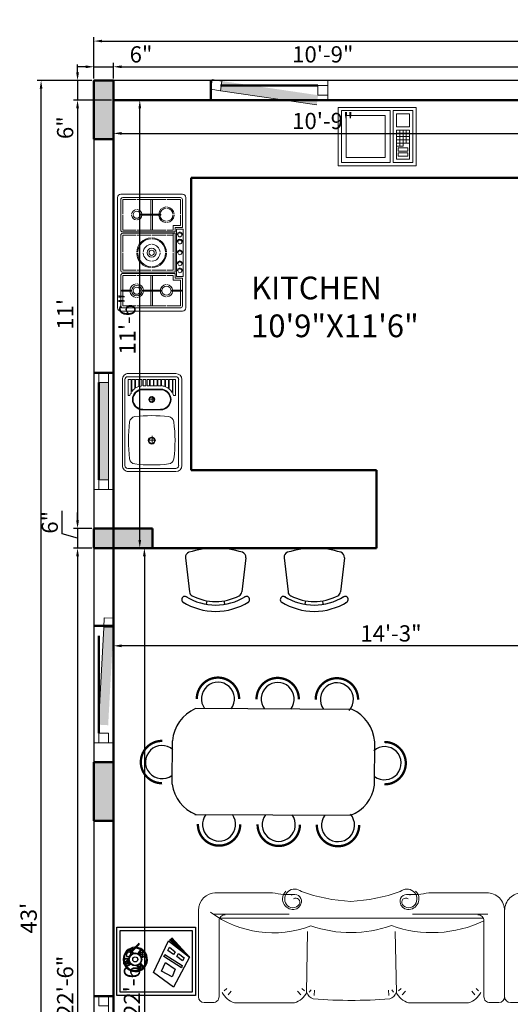
# Model space of a CAD drawing. Units: inches. Extents: x 3064 to 19385, y 846 to 15425.
# Tile 84 of 108: x 7077 to 7228, y 1112 to 1415. Entities that reach past the tile are written whole.
import ezdxf

# ---------------------------------------------------------------- set-up
doc = ezdxf.new("R2010")
doc.units = ezdxf.units.IN
for name, color, linetype, lineweight in [('A-ANNO-DIMS', 2, 'Continuous', 18), ('A-AREA-IDEN', 3, 'Continuous', 18), ('A-COLS', 1, 'Continuous', 35), ('A-EQPM', 8, 'Continuous', 18), ('A-FLOR-FIXT', 9, 'Continuous', 18), ('A-FURN', 8, 'Continuous', 18), ('A-GLAZ', 4, 'Continuous', 18), ('A-WALL', 7, 'Continuous', 50), ('C-PROP', 6, 'Continuous', 25)]:
    doc.layers.add(name, color=color, linetype=linetype, lineweight=lineweight)
for name, color, linetype in [('BLO', 135, 'Continuous'), ('FUR', 42, 'Continuous'), ('NOITHAT', 21, 'Continuous'), ('Win', 152, 'Continuous')]:
    doc.layers.add(name, color=color, linetype=linetype)
doc.styles.get("Standard").update_dxf_attribs({"font": 'arial.ttf'})
doc.dimstyles.new('ISO-25', dxfattribs={"dimtxt": 9, "dimasz": 2.5, "dimexe": 1.25, "dimexo": 0.625, "dimtad": 1, "dimdec": 1, "dimlunit": 3, "dimtxsty": 'Standard', "dimcen": 2.5, "dimadec": 0, "dimazin": 0, "dimtfac": 1, "dimtdec": 1, "dimtmove": 0, "dimatfit": 3, "dimfxl": 1, "dimarcsym": 0})

# ---------------------------------------------------------------- blocks, each defined once
blk = doc.blocks.new('*D291')
at = {"layer": 'A-ANNO-DIMS', "color": 0, "lineweight": -2, "transparency": 16777216}
for p, q in [((7099.71, 1396.96), (7099.71, 1401.84)), ((7105.71, 1396.96), (7105.71, 1401.84)), ((7097.21, 1400.59), (7094.71, 1400.59)), ((7099.71, 1400.59), (7105.71, 1400.59)), ((7108.21, 1400.59), (7117.73, 1400.59))]:
    blk.add_line(p, q, dxfattribs=at)
at = {"layer": 'A-ANNO-DIMS', "color": 0, "transparency": 16777216}
for points in [[(7097.21, 1401.01), (7097.21, 1400.18), (7099.71, 1400.59)], [(7108.21, 1401.01), (7108.21, 1400.18), (7105.71, 1400.59)]]:
    blk.add_solid(points, dxfattribs=at)
at = {"layer": 'Defpoints', "color": 0, "transparency": 16777216}
for p in [(7105.71, 1400.59), (7099.71, 1396.34), (7105.71, 1396.34)]:
    blk.add_point(p, dxfattribs=at)
at = {"layer": 'A-ANNO-DIMS', "color": 0, "transparency": 16777216, "insert": (7114.22, 1403.77), "char_height": 5, "attachment_point": 5}
blk.add_mtext('6"', dxfattribs=at)
blk = doc.blocks.new('*D292')
at = {"layer": 'A-ANNO-DIMS', "color": 0, "lineweight": -2, "transparency": 16777216}
for p, q in [((7105.71, 1396.96), (7105.71, 1401.84)), ((7234.71, 1396.96), (7234.71, 1401.84)), ((7108.21, 1400.59), (7232.21, 1400.59))]:
    blk.add_line(p, q, dxfattribs=at)
at = {"layer": 'A-ANNO-DIMS', "color": 0, "transparency": 16777216}
for points in [[(7108.21, 1401.01), (7108.21, 1400.18), (7105.71, 1400.59)], [(7232.21, 1401.01), (7232.21, 1400.18), (7234.71, 1400.59)]]:
    blk.add_solid(points, dxfattribs=at)
at = {"layer": 'Defpoints', "color": 0, "transparency": 16777216}
for p in [(7234.71, 1400.59), (7105.71, 1396.34), (7234.71, 1396.34)]:
    blk.add_point(p, dxfattribs=at)
at = {"layer": 'A-ANNO-DIMS', "color": 0, "transparency": 16777216, "insert": (7170.21, 1403.77), "char_height": 5, "attachment_point": 5}
blk.add_mtext('10\'-9"', dxfattribs=at)
blk = doc.blocks.new('*D296')
at = {"layer": 'A-ANNO-DIMS', "color": 0, "lineweight": -2, "transparency": 16777216}
for p, q in [((7094.68, 1398.84), (7094.68, 1401.34)), ((7099.08, 1396.34), (7093.43, 1396.34)), ((7094.68, 1396.34), (7094.68, 1390.34)), ((7105.08, 1390.34), (7093.43, 1390.34)), ((7094.68, 1387.84), (7094.68, 1378.32))]:
    blk.add_line(p, q, dxfattribs=at)
at = {"layer": 'A-ANNO-DIMS', "color": 0, "transparency": 16777216}
for points in [[(7094.26, 1398.84), (7095.09, 1398.84), (7094.68, 1396.34)], [(7094.26, 1387.84), (7095.09, 1387.84), (7094.68, 1390.34)]]:
    blk.add_solid(points, dxfattribs=at)
at = {"layer": 'Defpoints', "color": 0, "transparency": 16777216}
for p in [(7099.71, 1396.34), (7094.68, 1390.34), (7105.71, 1390.34)]:
    blk.add_point(p, dxfattribs=at)
at = {"layer": 'A-ANNO-DIMS', "color": 0, "transparency": 16777216, "insert": (7091.5, 1381.83), "char_height": 5, "attachment_point": 5, "rotation": 90}
blk.add_mtext('6"', dxfattribs=at)
blk = doc.blocks.new('*D297')
at = {"layer": 'A-ANNO-DIMS', "color": 0, "lineweight": -2, "transparency": 16777216}
for p, q in [((7105.08, 1390.34), (7093.43, 1390.34)), ((7094.68, 1387.84), (7094.68, 1260.84)), ((7099.08, 1258.34), (7093.43, 1258.34))]:
    blk.add_line(p, q, dxfattribs=at)
at = {"layer": 'A-ANNO-DIMS', "color": 0, "transparency": 16777216}
for points in [[(7094.26, 1387.84), (7095.09, 1387.84), (7094.68, 1390.34)], [(7094.26, 1260.84), (7095.09, 1260.84), (7094.68, 1258.34)]]:
    blk.add_solid(points, dxfattribs=at)
at = {"layer": 'Defpoints', "color": 0, "transparency": 16777216}
for p in [(7105.71, 1390.34), (7094.68, 1258.34), (7099.71, 1258.34)]:
    blk.add_point(p, dxfattribs=at)
at = {"layer": 'A-ANNO-DIMS', "color": 0, "transparency": 16777216, "insert": (7091.54, 1324.34), "char_height": 5, "attachment_point": 5, "rotation": 90}
blk.add_mtext("11'", dxfattribs=at)
blk = doc.blocks.new('*D298')
at = {"layer": 'A-ANNO-DIMS', "color": 0, "lineweight": -2, "transparency": 16777216}
for p, q in [((7089.94, 1256.76), (7089.94, 1263.79)), ((7094.68, 1260.84), (7094.68, 1263.34)), ((7094.68, 1255.34), (7089.94, 1256.76)), ((7099.08, 1258.34), (7093.43, 1258.34)), ((7094.68, 1258.34), (7094.68, 1252.34)), ((7094.68, 1258.34), (7094.68, 1252.34)), ((7099.08, 1252.34), (7093.43, 1252.34)), ((7094.68, 1249.84), (7094.68, 1247.34))]:
    blk.add_line(p, q, dxfattribs=at)
at = {"layer": 'A-ANNO-DIMS', "color": 0, "transparency": 16777216}
for points in [[(7094.26, 1260.84), (7095.09, 1260.84), (7094.68, 1258.34)], [(7094.26, 1249.84), (7095.09, 1249.84), (7094.68, 1252.34)]]:
    blk.add_solid(points, dxfattribs=at)
at = {"layer": 'Defpoints', "color": 0, "transparency": 16777216}
for p in [(7099.71, 1258.34), (7094.68, 1252.34), (7099.71, 1252.34)]:
    blk.add_point(p, dxfattribs=at)
at = {"layer": 'A-ANNO-DIMS', "color": 0, "transparency": 16777216, "insert": (7086.76, 1260.27), "char_height": 5, "attachment_point": 5, "rotation": 90}
blk.add_mtext('6"', dxfattribs=at)
blk = doc.blocks.new('*D299')
at = {"layer": 'A-ANNO-DIMS', "color": 0, "lineweight": -2, "transparency": 16777216}
for p, q in [((7099.08, 1252.34), (7093.43, 1252.34)), ((7094.68, 1249.84), (7094.68, 984.84)), ((7105.08, 982.34), (7093.43, 982.34))]:
    blk.add_line(p, q, dxfattribs=at)
at = {"layer": 'A-ANNO-DIMS', "color": 0, "transparency": 16777216}
for points in [[(7094.26, 1249.84), (7095.09, 1249.84), (7094.68, 1252.34)], [(7094.26, 984.84), (7095.09, 984.84), (7094.68, 982.34)]]:
    blk.add_solid(points, dxfattribs=at)
at = {"layer": 'Defpoints', "color": 0, "transparency": 16777216}
for p in [(7099.71, 1252.34), (7094.68, 982.34), (7105.71, 982.34)]:
    blk.add_point(p, dxfattribs=at)
at = {"layer": 'A-ANNO-DIMS', "color": 0, "transparency": 16777216, "insert": (7091.5, 1117.34), "char_height": 5, "attachment_point": 5, "rotation": 90}
blk.add_mtext('22\'-6"', dxfattribs=at)
blk = doc.blocks.new('*D303')
at = {"layer": 'A-ANNO-DIMS', "color": 0, "lineweight": -2, "transparency": 16777216}
for p, q in [((7099.08, 1396.34), (7082.19, 1396.34)), ((7083.44, 882.84), (7083.44, 1393.84)), ((7099.08, 880.34), (7082.19, 880.34))]:
    blk.add_line(p, q, dxfattribs=at)
at = {"layer": 'A-ANNO-DIMS', "color": 0, "transparency": 16777216}
for points in [[(7083.02, 1393.84), (7083.86, 1393.84), (7083.44, 1396.34)], [(7083.02, 882.84), (7083.86, 882.84), (7083.44, 880.34)]]:
    blk.add_solid(points, dxfattribs=at)
at = {"layer": 'Defpoints', "color": 0, "transparency": 16777216}
for p in [(7083.44, 1396.34), (7099.71, 1396.34), (7099.71, 880.34)]:
    blk.add_point(p, dxfattribs=at)
at = {"layer": 'A-ANNO-DIMS', "color": 0, "transparency": 16777216, "insert": (7080.26, 1138.34), "char_height": 5, "attachment_point": 5, "rotation": 90}
blk.add_mtext("43'", dxfattribs=at)
blk = doc.blocks.new('*D315')
at = {"layer": 'A-ANNO-DIMS', "color": 0, "lineweight": -2, "transparency": 16777216}
for p, q in [((7099.71, 1396.96), (7099.71, 1409.76)), ((7102.21, 1408.51), (7439.21, 1408.51)), ((7441.71, 1396.96), (7441.71, 1409.76))]:
    blk.add_line(p, q, dxfattribs=at)
at = {"layer": 'A-ANNO-DIMS', "color": 0, "transparency": 16777216}
for points in [[(7102.21, 1408.93), (7102.21, 1408.1), (7099.71, 1408.51)], [(7439.21, 1408.93), (7439.21, 1408.1), (7441.71, 1408.51)]]:
    blk.add_solid(points, dxfattribs=at)
at = {"layer": 'Defpoints', "color": 0, "transparency": 16777216}
for p in [(7441.71, 1408.51), (7099.71, 1396.34), (7441.71, 1396.34)]:
    blk.add_point(p, dxfattribs=at)
at = {"layer": 'A-ANNO-DIMS', "color": 0, "transparency": 16777216, "insert": (7270.71, 1411.69), "char_height": 5, "attachment_point": 5}
blk.add_mtext('28\'-6"', dxfattribs=at)
blk = doc.blocks.new('*D288')
at = {"layer": 'A-ANNO-DIMS', "color": 0, "lineweight": -2, "transparency": 16777216}
for p, q in [((7105.71, 1389.71), (7105.71, 1378.82)), ((7234.71, 1389.71), (7234.71, 1378.82)), ((7108.21, 1380.07), (7232.21, 1380.07))]:
    blk.add_line(p, q, dxfattribs=at)
at = {"layer": 'A-ANNO-DIMS', "color": 0, "transparency": 16777216}
for points in [[(7108.21, 1380.49), (7108.21, 1379.66), (7105.71, 1380.07)], [(7232.21, 1380.49), (7232.21, 1379.66), (7234.71, 1380.07)]]:
    blk.add_solid(points, dxfattribs=at)
at = {"layer": 'Defpoints', "color": 0, "transparency": 16777216}
for p in [(7105.71, 1390.34), (7234.71, 1390.34), (7234.71, 1380.07)]:
    blk.add_point(p, dxfattribs=at)
at = {"layer": 'A-ANNO-DIMS', "color": 0, "transparency": 16777216, "insert": (7170.21, 1383.25), "char_height": 5, "attachment_point": 5}
blk.add_mtext('10\'-9"', dxfattribs=at)
blk = doc.blocks.new('*D289')
at = {"layer": 'A-ANNO-DIMS', "color": 0, "lineweight": -2, "transparency": 16777216}
for p, q in [((7106.33, 1390.34), (7115.09, 1390.34)), ((7113.84, 1254.84), (7113.84, 1387.84)), ((7106.33, 1252.34), (7115.09, 1252.34))]:
    blk.add_line(p, q, dxfattribs=at)
at = {"layer": 'A-ANNO-DIMS', "color": 0, "transparency": 16777216}
for points in [[(7113.43, 1387.84), (7114.26, 1387.84), (7113.84, 1390.34)], [(7113.43, 1254.84), (7114.26, 1254.84), (7113.84, 1252.34)]]:
    blk.add_solid(points, dxfattribs=at)
at = {"layer": 'Defpoints', "color": 0, "transparency": 16777216}
for p in [(7105.71, 1390.34), (7113.84, 1390.34), (7105.71, 1252.34)]:
    blk.add_point(p, dxfattribs=at)
at = {"layer": 'A-ANNO-DIMS', "color": 0, "transparency": 16777216, "insert": (7110.67, 1321.34), "char_height": 5, "attachment_point": 5, "rotation": 90}
blk.add_mtext('11\'-6"', dxfattribs=at)
blk = doc.blocks.new('*D223')
at = {"layer": 'A-ANNO-DIMS', "color": 0, "lineweight": -2, "transparency": 16777216}
for p, q in [((7106.33, 1252.34), (7116.51, 1252.34)), ((7115.26, 1249.84), (7115.26, 984.84)), ((7106.33, 982.34), (7116.51, 982.34))]:
    blk.add_line(p, q, dxfattribs=at)
at = {"layer": 'A-ANNO-DIMS', "color": 0, "transparency": 16777216}
for points in [[(7114.84, 1249.84), (7115.67, 1249.84), (7115.26, 1252.34)], [(7114.84, 984.84), (7115.67, 984.84), (7115.26, 982.34)]]:
    blk.add_solid(points, dxfattribs=at)
at = {"layer": 'Defpoints', "color": 0, "transparency": 16777216}
for p in [(7105.71, 1252.34), (7105.71, 982.34), (7115.26, 982.34)]:
    blk.add_point(p, dxfattribs=at)
at = {"layer": 'A-ANNO-DIMS', "color": 0, "transparency": 16777216, "insert": (7112.08, 1117.34), "char_height": 5, "attachment_point": 5, "rotation": 90}
blk.add_mtext('22\'-6"', dxfattribs=at)
blk = doc.blocks.new('*D239')
at = {"layer": 'A-ANNO-DIMS', "color": 0, "lineweight": -2, "transparency": 16777216}
for p, q in [((7105.71, 1222.85), (7105.71, 1223.48)), ((7276.71, 1222.85), (7276.71, 1223.48)), ((7274.21, 1222.23), (7108.21, 1222.23))]:
    blk.add_line(p, q, dxfattribs=at)
at = {"layer": 'A-ANNO-DIMS', "color": 0, "transparency": 16777216}
for points in [[(7108.21, 1222.64), (7108.21, 1221.81), (7105.71, 1222.23)], [(7274.21, 1222.64), (7274.21, 1221.81), (7276.71, 1222.23)]]:
    blk.add_solid(points, dxfattribs=at)
at = {"layer": 'Defpoints', "color": 0, "transparency": 16777216}
for p in [(7105.71, 1222.23), (7105.71, 1222.23), (7276.71, 1222.23)]:
    blk.add_point(p, dxfattribs=at)
at = {"layer": 'A-ANNO-DIMS', "color": 0, "transparency": 16777216, "insert": (7191.21, 1225.4), "char_height": 5, "attachment_point": 5}
blk.add_mtext('14\'-3"', dxfattribs=at)
blk = doc.blocks.new('din')
at = {"layer": 'FUR', "ltscale": 0.25}
for p, q in [((70.23, 15.24), (9.28, 15.24)), ((0, 3.44), (0, -13.56)), ((79.14, 3.44), (79.14, -13.56)), ((8.91, -26.16), (70.23, -26.16))]:
    blk.add_line(p, q, dxfattribs=at)
at = {"layer": 'FUR', "ltscale": 0.25, "const_width": 0.9}
for points in [[(22.5, 19.02, 1.012537), (5.94, 19.02, 1.012537)], [(45.67, 19.02, 1.012537), (29.11, 19.02, 1.012537)], [(69.02, 19.02, 1.012537), (52.46, 19.02, 1.012537)], [(-3.79, 3.1, 1.012537), (-3.79, -13.47, 1.012537)], [(83.08, 3.1, -1.012537), (83.08, -13.47, -1.012537)], [(23.18, -29.95, -1.012537), (6.61, -29.95, -1.012537)], [(46.34, -29.95, -1.012537), (29.78, -29.95, -1.012537)], [(69.7, -29.95, -1.012537), (53.14, -29.95, -1.012537)]]:
    blk.add_lwpolyline(points, format="xyb", dxfattribs=at)
at = {"layer": 'FUR', "ltscale": 0.25}
for centre, radius, start, end in [((14.22, 19.13), 6.48, 323.1301, 221.2163), ((37.39, 19.13), 6.48, 323.1301, 216.8699), ((60.74, 19.13), 6.48, 323.1301, 216.8699), ((14.55, 1.54), 14.67, 111.0491, 172.5731), ((64.59, 1.54), 14.67, 7.4269, 68.9509), ((-3.89, -5.18), 6.48, 53.1301, 311.2163), ((83.18, -5.18), 6.48, 228.7837, 126.8699), ((15.28, -12.21), 15.34, 185.0602, 245.4675), ((63.86, -12.21), 15.34, 294.5325, 354.9398), ((14.89, -30.05), 6.48, 138.7837, 36.8699), ((38.06, -30.05), 6.48, 143.1301, 36.8699), ((61.42, -30.05), 6.48, 143.1301, 36.8699)]:
    blk.add_arc(centre, radius, start, end, dxfattribs=at)
blk = doc.blocks.new('A$C558E769F')
at = {"layer": 'NOITHAT'}
for p, q in [((29.4, 426.4), (61.1, 154.1)), ((508.9, 426.4), (477.2, 154.1)), ((197.1, 55.9), (201.8, 84.2)), ((341.2, 55.9), (336.5, 84.2))]:
    blk.add_line(p, q, dxfattribs=at)
for centre, radius, start, end in [((69.1, 431), 40, 107.02981, 186.63805), ((269.2, -222), 723, 72.97019, 107.02981), ((469.2, 431), 40, 353.36195, 72.97019), ((25.3, 93.7), 25.7, 44.80366, 252.32262), ((269.2, 492.6), 442.6, 237.77056, 302.22944), ((100.8, 158.7), 40, 186.63805, 243.24485), ((269.2, 492.6), 413.9, 243.24485, 296.75515), ((437.5, 158.7), 40, 296.75515, 353.36195), ((513, 93.7), 25.7, 287.67738, 135.19634), ((269.2, 492.6), 492.6, 237.85101, 302.14899)]:
    blk.add_arc(centre, radius, start, end, dxfattribs=at)
blk = doc.blocks.new('sofa-32')
at = {"color": 0, "linetype": 'ByBlock'}
for p, q in [((-0.026, 0.9238), (-0.1, 0.9238)), ((0.657, 0.9252), (0.1531, 0.9252)), ((1.6158, 0.9252), (2.1197, 0.9252)), ((2.3728, 0.9238), (2.2988, 0.9238)), ((-0.15, 0.15), (-0.15, 0.8738)), ((0.024, 0.2361), (0.024, 0.8738)), ((0.05, 0.8375), (0.05, 0.8379)), ((0.1006, 0.8574), (0.1265, 0.8286)), ((0.7096, 0.8574), (0.6837, 0.8286)), ((0.7682, 0.3257), (0.7597, 0.8384)), ((0.7601, 0.8375), (0.7601, 0.8379)), ((0.7823, 0.8346), (0.7966, 0.8162)), ((0.8227, 0.8633), (0.8259, 0.8195)), ((1.4501, 0.8633), (1.447, 0.8195)), ((1.4906, 0.8346), (1.4762, 0.8162)), ((1.5046, 0.3257), (1.5131, 0.8384)), ((1.5127, 0.8375), (1.5127, 0.8379)), ((1.5632, 0.8574), (1.5891, 0.8286)), ((2.1722, 0.8574), (2.1463, 0.8286)), ((2.2228, 0.8375), (2.2228, 0.8379)), ((2.2228, 0.8375), (2.2228, 0.8379)), ((2.2488, 0.2361), (2.2488, 0.8738)), ((2.4228, 0.15), (2.4228, 0.8738)), ((0.0903, 0.8062), (0.0682, 0.8242)), ((0.7199, 0.8062), (0.742, 0.8242)), ((1.5529, 0.8062), (1.5308, 0.8242)), ((2.1825, 0.8062), (2.2046, 0.8242)), ((-0.01, 0.1801), (0.6238, 0.1801)), ((0.0289, 0.2145), (2.2439, 0.2145)), ((2.2948, 0.1801), (1.661, 0.1801)), ((0, 0), (0.4856, 0)), ((2.2848, 0), (1.7991, 0))]:
    blk.add_line(p, q, dxfattribs=at)
at = {"color": 0, "linetype": 'ByBlock', "extrusion": (0, 0, -1)}
for centre, major_axis, start_param, end_param in [((-0.1, 0.8738), (0.0354, 0.0354), 3.926992, 5.497787), ((-0.026, 0.8738), (-0.0354, 0.0354), 0.785398, 2.356196), ((0.1997, 0.7661), (0.1173, 0.1173), 4.372209, 5.213218), ((0.6105, 0.7661), (0.1173, 0.1173), -0.500829, 0.34018), ((1.6624, 0.7661), (0.1173, 0.1173), 4.372209, 5.213218), ((2.0731, 0.7661), (-0.1173, 0.1173), 1.069968, 1.910976), ((2.2988, 0.8738), (-0.0354, 0.0354), 5.497786, 7.068583), ((2.3728, 0.8738), (0.0354, 0.0354), -0.785398, 0.785398), ((0.8378, 0.8143), (-0.0573, 0.0573), 5.78837, 6.779907), ((1.1202, -2.7856), (2.6094, 2.6094), -0.86827, -0.778364), ((1.1526, -2.7856), (2.6094, 2.6094), -0.792432, -0.702526), ((1.435, 0.8143), (-0.0573, 0.0573), 1.074075, 2.065611), ((0.4599, -0.6685), (0.71, 0.71), 5.048761, 5.844539), ((1.1424, -0.6685), (-0.71, 0.71), 0.438646, 1.125824), ((1.7954, -0.5466), (-0.6249, 0.6249), 0.417642, 1.423136), ((0.074, 0.2361), (0.0354, 0.0354), 2.356194, 3.926992), ((2.1988, 0.2361), (0.0354, 0.0354), 0.785397, 2.356194), ((0, 0.15), (0.1061, 0.1061), 2.356194, 3.926992), ((0.6576, 0.0525), (-0.0624, 0.0624), 4.675944, 7.152385), ((0.6708, 0.0524), (-0.059, 0.059), 3.186406, 6.094039), ((0.6552, 0.0629), (0.0458, 0.0458), 4.523242, 6.472337), ((0.6801, 0.0798), (-0.0245, 0.0245), 1.759948, 4.523241), ((0.6592, 0.0712), (-0.0491, 0.0491), 0.8692, 2.230507), ((1.6256, 0.0712), (-0.0491, 0.0491), 5.623477, 6.984784), ((1.614, 0.0524), (0.059, 0.059), 0.189149, 3.096782), ((1.6047, 0.0798), (0.0245, 0.0245), 1.759947, 4.52324), ((1.6295, 0.0629), (0.0458, 0.0458), 4.52324, 6.472335), ((1.6271, 0.0525), (-0.0624, 0.0624), 0.701599, 3.17804), ((2.2728, 0.15), (0.1061, 0.1061), 0.785398, 2.356194), ((0.6324, -0.6613), (-0.479, 0.479), 0.566947, 0.842011), ((0.6701, 0.0726), (0.0414, 0.0414), 0.659711, 2.852687), ((1.2153, -1.3904), (1.0359, 1.0359), 5.158011, 5.447964), ((1.0694, -1.3904), (1.0359, 1.0359), 5.547613, 5.837566), ((1.6147, 0.0726), (-0.0414, 0.0414), 3.430501, 5.623477), ((1.6523, -0.6613), (0.479, 0.479), 5.441177, 5.716241)]:
    blk.add_ellipse(centre, major_axis=major_axis, ratio=1, start_param=start_param, end_param=end_param, dxfattribs=at)
blk = doc.blocks.new('sofa-34')
at = {"color": 0, "linetype": 'ByBlock'}
for p, q in [((-0.026, 0.9238), (-0.1, 0.9238)), ((0.657, 0.9252), (0.1531, 0.9252)), ((0.8361, 0.9238), (0.9101, 0.9238)), ((-0.15, 0.15), (-0.15, 0.8738)), ((0.024, 0.2361), (0.024, 0.8738)), ((0.05, 0.8375), (0.05, 0.8379)), ((0.1006, 0.8574), (0.1265, 0.8286)), ((0.7096, 0.8574), (0.6837, 0.8286)), ((0.7601, 0.8375), (0.7601, 0.8379)), ((0.7602, 0.8375), (0.7601, 0.8379)), ((0.7861, 0.2361), (0.7861, 0.8738)), ((0.9601, 0.15), (0.9601, 0.8738)), ((0.0903, 0.8062), (0.0682, 0.8242)), ((0.7199, 0.8062), (0.742, 0.8242)), ((-0.01, 0.1801), (0.2738, 0.1801)), ((0.0289, 0.2145), (0.7812, 0.2145)), ((0.8201, 0.1801), (0.5364, 0.1801))]:
    blk.add_line(p, q, dxfattribs=at)
blk.add_arc((0.4051, 0.1479), 0.2579, 40.79835, 139.20165, dxfattribs=at)
at = {"color": 0, "linetype": 'ByBlock', "extrusion": (0, 0, -1)}
for centre, major_axis, ratio, start_param, end_param in [((-0.1, 0.8738), (0.0354, 0.0354), 1, 3.926992, 5.497787), ((-0.026, 0.8738), (-0.0354, 0.0354), 1, 0.785398, 2.356196), ((0.1997, 0.7661), (0.1173, 0.1173), 1, 4.372209, 5.213218), ((0.6105, 0.7661), (0.1173, 0.1173), 1, -0.500829, 0.34018), ((0.5004, -0.5869), (-0.4145, 0.931), 0.264583, -0.381915, 0.387685), ((0.074, 0.2361), (-0.0354, 0.0354), 1, 3.926991, 5.497788), ((0, 0.15), (0.1061, 0.1061), 1, 2.356194, 3.926992), ((0.1167, 0.0525), (-0.0624, 0.0624), 1, 4.675944, 7.152385), ((0.1299, 0.0524), (-0.059, 0.059), 1, 3.186406, 6.094039), ((0.1144, 0.0629), (-0.0458, 0.0458), 1, 6.094039, 8.043134), ((0.1392, 0.0798), (0.0245, 0.0245), 1, 0.189152, 2.952444), ((0.1183, 0.0712), (0.0491, 0.0491), 1, -0.701597, 0.659711), ((0.179, -0.6576), (-0.2506, 0.635), 0.885019, 0.124301, 0.339591), ((0.1292, 0.0726), (-0.0414, 0.0414), 1, 2.230507, 4.423483), ((0.3517, -0.5578), (0.7346, 0.1067), 0.76838, 4.597815, 5.20076)]:
    blk.add_ellipse(centre, major_axis=major_axis, ratio=ratio, start_param=start_param, end_param=end_param, dxfattribs=at)
at = {"color": 0, "linetype": 'ByBlock'}
for centre, major_axis, ratio, start_param, end_param in [((0.8361, 0.8738), (0.0354, 0.0354), 1, 0.785398, 2.356196), ((0.9101, 0.8738), (-0.0354, 0.0354), 1, 3.926992, 5.497787), ((0.3097, -0.5869), (0.4145, 0.931), 0.264583, -0.381915, 0.387685), ((0.7361, 0.2361), (0.0354, 0.0354), 1, 3.926991, 5.497788), ((0.6918, 0.0712), (-0.0491, 0.0491), 1, -0.701597, 0.659711), ((0.6802, 0.0524), (0.059, 0.059), 1, 3.186406, 6.094039), ((0.6709, 0.0798), (-0.0245, 0.0245), 1, 0.189152, 2.952444), ((0.6958, 0.0629), (0.0458, 0.0458), 1, 6.094039, 8.043134), ((0.6934, 0.0525), (0.0624, 0.0624), 1, 4.675944, 7.152385), ((0.8101, 0.15), (-0.1061, 0.1061), 1, 2.356194, 3.926992), ((0.6809, 0.0726), (0.0414, 0.0414), 1, 2.230507, 4.423483), ((0.6312, -0.6576), (0.2506, 0.635), 0.885019, 0.124301, 0.339591)]:
    blk.add_ellipse(centre, major_axis=major_axis, ratio=ratio, start_param=start_param, end_param=end_param, dxfattribs=at)
blk = doc.blocks.new('sink 1')
for points in [[(-7.34, 1.48), (-7.34, 22.73)], [(-6.56, 1.48), (-6.56, 22.73)], [(5.86, 24.22), (-5.86, 24.22)], [(6.01, 23.43), (-5.86, 23.43)], [(6.72, 1.48), (6.72, 22.73)], [(7.34, 1.48), (7.34, 22.73)], [(0, 15.39), (0, 17.42)], [(1.09, 16.48), (-0.94, 16.48)], [(-2.09, 8.99), (2.28, 8.99)], [(-2.09, 8.84), (2.28, 8.84)], [(-5.78, 5.39), (-5.78, 5.39)], [(-5.31, 5.39), (-5.31, 5.39)], [(-5.16, 4.92), (-5.16, 4.92)], [(0.78, 6.33), (-0.78, 6.33)], [(0, 5.55), (0, 7.26)], [(5.16, 4.92), (5.16, 4.92)], [(5.94, 5.39), (5.94, 5.39)], [(-5, 1.48), (-5, 4.69)], [(-5, 1.48), (-4.22, 1.48), (-4.22, 3.83)], [(-4.84, 4.45), (-4.84, 4.45)], [(-4.22, 3.83), (-4.22, 3.83)], [(-4.06, 1.48), (-4.06, 3.69)], [(-4.06, 1.48), (-3.28, 1.48), (-3.28, 3.27)], [(-3.91, 3.52), (-3.91, 3.52)], [(-3.28, 3.2), (-3.28, 3.2)], [(-3.12, 3.2), (-3.12, 3.2)], [(-2.34, 3.05), (-2.34, 3.05)], [(-2.19, 3.05), (-2.19, 3.05)], [(-2.09, 3.99), (2.28, 3.99)], [(-2.09, 3.84), (2.28, 3.84)], [(-1.41, 3.05), (-1.41, 3.05)], [(-1.25, 3.05), (-1.25, 3.05)], [(-0.47, 1.48), (-1.25, 1.48), (-1.25, 3.05), (-0.47, 3.05)], [(-0.62, 3.05), (-0.62, 3.05)], [(-0.47, 1.48), (-0.47, 3.05)], [(-0.31, 3.05), (-0.31, 3.05)], [(0.47, 1.48), (-0.31, 1.48), (-0.31, 3.05), (0.47, 3.05)], [(0.31, 3.05), (0.31, 3.05)], [(0.47, 1.48), (0.47, 3.05)], [(0.62, 3.05), (0.62, 3.05)], [(1.25, 3.05), (1.25, 3.05)], [(1.56, 3.05), (1.56, 3.05)], [(2.19, 3.05), (2.19, 3.05)], [(2.5, 3.05), (2.5, 3.05)], [(3.12, 3.2), (3.12, 3.2)], [(3.28, 1.48), (4.06, 1.48), (4.06, 3.57)], [(3.28, 1.48), (3.28, 3.2)], [(3.44, 3.2), (3.44, 3.2)], [(4.06, 3.52), (4.06, 3.52)], [(4.22, 1.48), (4.22, 3.67)], [(4.37, 3.83), (4.37, 3.83)], [(5, 4.45), (5, 4.45)], [(6.01, 0.78), (-5.86, 0.78)], [(5.86, 0), (-5.86, 0)], [(-5.78, 1.48), (-5.78, 1.48)], [(-5.16, 1.48), (-5.16, 1.48)], [(-4.84, 1.48), (-4.84, 1.48)], [(-4.22, 1.48), (-4.22, 1.48)], [(-3.91, 1.48), (-3.91, 1.48)], [(-3.28, 1.48), (-3.28, 1.48)], [(-3.12, 1.48), (-3.12, 1.48)], [(-2.34, 1.48), (-2.34, 1.48)], [(-2.19, 1.48), (-2.19, 1.48)], [(-1.41, 1.48), (-1.41, 1.48)], [(-1.25, 1.48), (-1.25, 1.48)], [(-0.62, 1.48), (-0.62, 1.48)], [(-0.31, 1.48), (-0.31, 1.48)], [(0.31, 1.48), (0.31, 1.48)], [(0.62, 1.48), (0.62, 1.48)], [(1.25, 1.48), (1.25, 1.48)], [(1.56, 1.48), (1.56, 1.48)], [(2.19, 1.48), (2.19, 1.48)], [(2.5, 1.48), (2.5, 1.48)], [(3.12, 1.48), (3.12, 1.48)], [(3.44, 1.48), (3.44, 1.48)], [(4.06, 1.48), (4.06, 1.48)], [(4.37, 1.48), (4.37, 1.48)], [(5, 1.48), (5, 1.48)], [(5.16, 1.48), (5.16, 1.48)], [(5.94, 1.48), (5.94, 1.48)]]:
    blk.add_lwpolyline(points)
for points in [[(-5.16, 4.92), (-5.16, 1.48), (-5.78, 1.48), (-5.78, 5.39), (-5.31, 5.39, -0.068511), (-5.16, 4.92)], [(5.16, 4.92, 0.248301), (5.47, 5.39), (5.94, 5.39), (5.94, 1.48), (5.16, 1.48), (5.16, 4.92)], [(4.06, 3.57, -0.061679), (3.32, 3.22)], [(4.22, 1.48), (5, 1.48), (5, 4.45, -0.083542), (4.22, 3.67, -0.083542)]]:
    blk.add_lwpolyline(points, format="xyb")
for points in [[(-3.12, 3.22), (-3.12, 1.48), (-2.34, 1.48), (-2.34, 3.05, -0.06228)], [(2.5, 3.05), (2.5, 1.48), (3.12, 1.48), (3.12, 3.2, -0.050256)]]:
    blk.add_lwpolyline(points, format="xyb", close=True)
for points in [[(-2.19, 3.05), (-1.41, 3.05), (-1.41, 1.48), (-2.19, 1.48)], [(0.62, 3.05), (1.25, 3.05), (1.25, 1.48), (0.62, 1.48)], [(2.19, 1.48), (2.19, 3.05), (1.56, 3.05), (1.56, 1.48)]]:
    blk.add_lwpolyline(points, close=True)
for centre, radius in [((0.09, 16.57), 0.859), ((0.09, 16.57), 0.703), ((0.09, 6.41), 0.703), ((0.09, 6.41), 0.547)]:
    blk.add_circle(centre, radius)
for centre, radius, start, end in [((-5.86, 22.73), 1.48, 90, 180), ((-5.86, 22.73), 0.703, 90, 180), ((-3.87, 20.82), 1.53, 97.3256, 171.1849), ((0.09, -12.65), 35.23, 83.2159, 96.7841), ((4.06, 20.82), 1.53, 8.8151, 82.6744), ((5.86, 22.73), 1.48, 360, 90), ((6.01, 22.73), 0.703, 0, 90), ((30.19, 16.56), 35.85, 172.7947, 187.4213), ((-30, 16.56), 35.85, 352.5787, 7.2053), ((-3.89, 12.12), 1.48, 187.4212, 263.2159), ((0.09, 45.63), 35.23, 263.2159, 276.7841), ((4.08, 12.12), 1.48, 276.7841, 352.5788), ((-2.1, 6.41), 2.58, 90, 270), ((-2.1, 6.41), 2.42, 90, 270), ((2.28, 6.41), 2.58, 270, 90), ((2.28, 6.41), 2.42, 270, 90), ((-2.15, 6.48), 3.36, 212.1095, 232.0862), ((-2.1, 6.41), 3.36, 234.156, 249.3275), ((2.14, 6.36), 3.36, 289.8633, 290.5971), ((-5.86, 1.48), 1.48, 180, 270), ((-5.86, 1.48), 0.703, 180, 270), ((5.86, 1.48), 1.48, 270, 0), ((6.01, 1.48), 0.703, 270, 360)]:
    blk.add_arc(centre, radius, start, end)
blk = doc.blocks.new('STOVE')
for p, q in [((11.85, 19.7), (11.55, 19.7)), ((11.55, 16.92), (11.55, 19.7)), ((11.85, 16.92), (11.85, 19.7)), ((11.85, 16.92), (11.55, 16.92)), ((-11.85, 13.73), (-11.85, 7.62)), ((-11.85, 13.73), (-11.55, 13.73)), ((-11.55, 13.73), (-11.55, 7.62)), ((11.85, 13.23), (11.55, 13.23)), ((11.55, 13.23), (11.55, 7.57)), ((11.85, 13.23), (11.85, 7.57)), ((-11.85, 10.75), (-16.4, 10.75)), ((-11.85, 10.25), (-16.4, 10.25)), ((-7, 10.75), (-11.55, 10.75)), ((-7, 10.25), (-11.55, 10.25)), ((7, 10.75), (11.55, 10.75)), ((7, 10.25), (11.55, 10.25)), ((11.85, 10.75), (16.4, 10.75)), ((11.85, 10.25), (16.4, 10.25)), ((-11.85, 7.62), (-11.55, 7.62)), ((11.85, 7.57), (11.55, 7.57)), ((-7, 3.9), (-8.4, 3.9)), ((-7.8, 3.3), (-7.8, 1)), ((-6.4, 3.3), (-7.8, 3.3)), ((-5.4, 3.9), (-6, 3.9)), ((-5.4, 3.9), (-0.15, 3.9)), ((0.15, 3.9), (5.4, 3.9)), ((6.4, 3.3), (7.8, 3.3)), ((7, 3.9), (8.4, 3.9)), ((7.8, 3.3), (7.8, 1)), ((8.4, 3.9), (8.4, 1.6)), ((11.85, 4.28), (11.55, 4.28)), ((11.55, 4.28), (11.55, 1.3)), ((11.85, 4.28), (11.85, 1.3)), ((7.3, 2.8), (-7.3, 2.8)), ((-7.3, 2.8), (-7.3, 0.8)), ((7.3, 0.8), (-7.3, 0.8)), ((7.3, 2.8), (7.3, 0.8)), ((11.85, 1.3), (11.55, 1.3))]:
    blk.add_line(p, q)
for points in [[(-17, 21), (17, 21, -0.414214), (18, 20), (18, 1, -0.414214), (17, 0), (-17, 0, -0.414214), (-18, 1), (-18, 20, -0.414214)], [(6, 3.3), (-6, 3.3), (-6, 19.4, -0.414214), (-5.4, 20), (5.4, 20, -0.414214), (6, 19.4)]]:
    blk.add_lwpolyline(points, format="xyb", close=True)
for points in [[(-7.8, 1), (-16.4, 1, -0.414214), (-17, 1.6), (-17, 19.4, -0.414214), (-16.4, 20), (-7, 20, -0.414214), (-6.4, 19.4), (-6.4, 3.3)], [(6.4, 19.4, -0.414214), (7, 20), (16.4, 20, -0.414214), (17, 19.4), (17, 1.6, -0.414214), (16.4, 1), (7.8, 1)]]:
    blk.add_lwpolyline(points, format="xyb")
for points in [[(-16.4, 15.22), (-16.4, 19.4), (-11.85, 19.4)], [(-11.55, 19.4), (-7, 19.4), (-7, 15.22)], [(-5.4, 15.22), (-5.4, 19.4), (-0.15, 19.4)], [(0.15, 19.4), (5.4, 19.4), (5.4, 15.22)], [(6.4, 3.3), (6.4, 19.4)], [(7, 15.22), (7, 19.4), (11.55, 19.4)], [(11.85, 19.4), (16.4, 19.4), (16.4, 15.22)], [(-16.4, 6.08), (-16.4, 14.92)], [(-7, 14.92), (-7, 6.08)], [(-5.4, 10.65), (-5.4, 14.92)], [(5.4, 14.92), (5.4, 10.65)], [(7, 6.08), (7, 14.92)], [(16.4, 14.92), (16.4, 6.08)], [(-5.4, 6.08), (-5.4, 10.35)], [(5.4, 10.35), (5.4, 6.08)], [(-11.85, 1.6), (-16.4, 1.6), (-16.4, 5.77)], [(-8.4, 3.9), (-8.4, 1.6), (-11.55, 1.6)], [(-7, 5.77), (-7, 3.9)], [(-5.4, 3.9), (-5.4, 5.77)], [(5.4, 5.77), (5.4, 3.9)], [(7, 3.9), (7, 5.77)], [(16.4, 5.77), (16.4, 1.6), (11.85, 1.6)], [(11.55, 1.6), (8.4, 1.6)]]:
    blk.add_lwpolyline(points)
for centre, radius in [((-11.7, 15.07), 1.1), ((11.7, 15.07), 1.6), ((11.7, 15.07), 1.1), ((0, 10.5), 1.4), ((0, 10.5), 0.8), ((11.7, 5.93), 1.4), ((-5.49, 1.8), 0.6), ((-3.3, 1.8), 0.6), ((0, 1.8), 0.6), ((3.39, 1.8), 0.6), ((5.57, 1.8), 0.6)]:
    blk.add_circle(centre, radius)
for centre, radius, start, end in [((-11.7, 15.07), 1.6, 95.3794, 174.6206), ((-11.7, 15.07), 1.6, 5.3794, 84.6206), ((11.7, 15.07), 2.1, 94.096, 175.904), ((11.7, 15.07), 2.1, 4.096, 85.904), ((-11.7, 15.07), 1.6, 185.3794, 264.6206), ((-11.7, 15.07), 1.6, 275.3794, 354.6206), ((0, 10.5), 4.6, 91.8687, 178.1313), ((0, 10.5), 4.3, 91.9991, 178.0009), ((0, 10.5), 2.6, 93.3074, 176.6926), ((0, 10.5), 4.6, 1.8687, 88.1313), ((0, 10.5), 4.3, 1.9991, 88.0009), ((0, 10.5), 2.6, 3.3074, 86.6926), ((11.7, 15.07), 2.1, 184.096, 265.904), ((11.7, 15.07), 2.1, 274.096, 355.904), ((0, 10.5), 4.6, 181.8687, 268.1313), ((0, 10.5), 4.3, 181.9991, 268.0009), ((0, 10.5), 2.6, 183.3074, 266.6926), ((0, 10.5), 4.6, 271.8687, 358.1313), ((0, 10.5), 4.3, 271.9991, 358.0009), ((0, 10.5), 2.6, 273.3074, 356.6926), ((-11.7, 5.93), 2.4, 93.5833, 176.4167), ((-11.7, 5.93), 2, 94.3012, 175.6988), ((-11.7, 5.93), 2.4, 3.5833, 86.4167), ((-11.7, 5.93), 2, 4.3012, 85.6988), ((11.7, 5.93), 1.9, 94.5281, 175.4719), ((11.7, 5.93), 1.9, 4.5281, 85.4719), ((-11.7, 5.93), 2.4, 183.5833, 266.4167), ((-11.7, 5.93), 2, 184.3012, 265.6988), ((-11.7, 5.93), 2.4, 273.5833, 356.4167), ((-11.7, 5.93), 2, 274.3012, 355.6988), ((11.7, 5.93), 1.9, 184.5281, 265.4719), ((11.7, 5.93), 1.9, 274.5281, 355.4719), ((-5.49, 1.8), 0.846, 89.9979, 270), ((-3.3, 1.8), 0.846, 89.9979, 270), ((0, 1.8), 0.846, 89.9979, 270), ((3.39, 1.8), 0.846, 89.9979, 270), ((5.57, 1.8), 0.846, 89.9979, 270)]:
    blk.add_arc(centre, radius, start, end)
blk = doc.blocks.new('Microwave')
for p, q in [((18, 10), (22, 10)), ((19, 7), (19, 11)), ((20, 11), (20, 7)), ((21, 7), (21, 11)), ((22, 9), (18, 9)), ((18, 8), (22, 8)), ((22, 7), (18, 7)), ((19, 6), (19, 7)), ((20, 7), (20, 6)), ((20, 6), (18, 6))]:
    blk.add_line(p, q)
for points in [[(0, 0), (0, 18), (24, 18), (24, 0)], [(1, 1), (1, 17), (16, 17), (16, 1)], [(2.5, 2.5), (2.5, 15.5), (14.5, 15.5), (14.5, 2.5)], [(17, 1), (17, 17), (23, 17), (23, 1)], [(18, 12), (18, 16), (22, 16), (22, 12)], [(18, 2), (18, 11), (22, 11), (22, 2)], [(18.5, 4.5), (18.5, 5.5), (21.5, 5.5), (21.5, 4.5)], [(18.5, 3), (18.5, 4), (21.5, 4), (21.5, 3)]]:
    blk.add_lwpolyline(points, close=True)
blk = doc.blocks.new('ST1')
at = {"layer": 'BLO'}
for p, q in [((2.87, 1.65), (2.87, 24.72)), ((2.87, 24.72), (22.87, 24.72)), ((3.87, 2.65), (3.87, 23.72)), ((3.87, 23.72), (21.87, 23.72)), ((21.87, 23.72), (21.87, 2.65)), ((22.87, 24.72), (22.87, 1.65)), ((22.87, 1.65), (2.87, 1.65)), ((21.87, 2.65), (3.87, 2.65))]:
    blk.add_line(p, q, dxfattribs=at)
at = {"layer": 'Win'}
for p, q in [((11.4, 21.86), (12.09, 20.65)), ((11.51, 21.94), (12.19, 20.74)), ((11.57, 21.85), (13.19, 21.3)), ((12.55, 22.44), (12.13, 20.85)), ((12.55, 22.44), (13.25, 21.19)), ((12.69, 22.48), (13.4, 21.2)), ((14.51, 20.87), (14.54, 20.9)), ((14.64, 20.77), (14.67, 20.79)), ((15.43, 20.61), (15.22, 19.97)), ((15.22, 19.97), (15.71, 20.33)), ((15.27, 19.81), (15.82, 20.21)), ((15.37, 21.5), (15.64, 21.7)), ((15.41, 20.64), (17.8, 18.17)), ((15.46, 21.36), (15.76, 21.58)), ((15.54, 20.8), (16.34, 20.79)), ((15.54, 20.77), (18.02, 18.4)), ((15.76, 21.58), (15.55, 20.96)), ((17.88, 18.31), (15.58, 20.6)), ((15.87, 20.45), (16.34, 20.79)), ((15.99, 20.33), (16.41, 20.64)), ((10.46, 17.93), (11.6, 18.76)), ((10.53, 17.78), (11.65, 18.59)), ((10.53, 17.78), (12.23, 17.8)), ((11.59, 18.54), (11.11, 16.99)), ((11.11, 16.99), (12.23, 17.8)), ((11.23, 16.87), (12.37, 17.7)), ((13.9, 17.44), (14.58, 16.23)), ((14.03, 17.48), (14.71, 16.28)), ((14.09, 17.38), (15.67, 16.91)), ((15.04, 18.04), (14.71, 16.28)), ((14.97, 18.16), (15.67, 16.91)), ((15, 18.22), (15.87, 17.69)), ((15.13, 18.43), (16.01, 17.9)), ((15.14, 18.13), (15.77, 17.01)), ((5.28, 8.07), (9.58, 13.93)), ((8.3, 8.54), (10.02, 11.57)), ((9.58, 13.93), (18.91, 9.59)), ((10.02, 11.57), (12.5, 10.4)), ((12.5, 10.4), (10.58, 7.59)), ((10.98, 5.74), (14.34, 10.89)), ((14.87, 10.68), (11.67, 5.58)), ((18.91, 9.59), (14.09, 3.45)), ((14.09, 3.45), (19.17, 9.31)), ((14.09, 3.45), (19.44, 9.01)), ((14.09, 3.45), (19.64, 8.8)), ((14.34, 10.89), (14.87, 10.68)), ((14.86, 8.07), (16.06, 9.73)), ((17.01, 9.23), (15.7, 7.6)), ((16.06, 9.73), (17.01, 9.23)), ((14.09, 3.45), (5.28, 8.07)), ((10.58, 7.59), (8.3, 8.54)), ((13.06, 5.5), (14.27, 7.16)), ((15.21, 6.66), (13.91, 5.03)), ((14.09, 3.45), (19.77, 8.63)), ((14.27, 7.16), (15.21, 6.66)), ((15.7, 7.6), (14.86, 8.07)), ((11.67, 5.58), (10.98, 5.74)), ((13.91, 5.03), (13.06, 5.5))]:
    blk.add_line(p, q, dxfattribs=at)
for radius in [1.91, 1.75, 0.74]:
    blk.add_circle((13.43, 19.29), radius, dxfattribs=at)
for centre, radius, start, end in [((13.43, 19.29), 3.56, 1.5005, 355.5882), ((13.43, 19.29), 3.27, 6.8421, 0.252), ((15.21, 21.57), 0.956, 171.718, 281.8824), ((14.47, 21.69), 0.203, 96.3605, 174.3012), ((14.6, 20.95), 0.956, 349.0729, 98.9437), ((15.51, 20.66), 0.106, 78.1124, 194.2793), ((15.97, 17.77), 0.128, 220.7943, 60.0122), ((17.91, 18.29), 0.161, 227.8642, 43.7153)]:
    blk.add_arc(centre, radius, start, end, dxfattribs=at)
blk = doc.blocks.new('WIN-900-A')
h = blk.add_hatch(color=256)
h.dxf.hatch_style = 1
h.paths.add_polyline_path([(33, 0), (33, 3), (3, 3), (3, 0)])
blk.add_line((3, 0), (33, 0))
blk.add_lwpolyline([(3, 0), (0, 0), (0, 3), (3, 3)], close=True)
blk = doc.blocks.new('WIN-900')
blk.add_line((0, 0), (30, 0))
blk.add_lwpolyline([(30, 0), (30, 3), (33, 3), (33, 0)], close=True)
blk = doc.blocks.new('WIN-1900')
blk.add_line((3, 0), (3, 66))
blk.add_lwpolyline([(3, 66), (0, 66), (0, 69), (3, 69)], close=True)

msp = doc.modelspace()

# ---------------------------------------------------------------- hatches: boundary and pattern name
at = {"layer": 'A-COLS'}
h = msp.add_hatch(color=256, dxfattribs=at)
h.dxf.hatch_style = 1
h.paths.add_polyline_path([(7099.71, 1378.34), (7105.71, 1378.34), (7105.71, 1396.34), (7099.71, 1396.34)])
h = msp.add_hatch(color=256, dxfattribs=at)
h.dxf.hatch_style = 1
h.paths.add_polyline_path([(7117.71, 1252.34), (7117.71, 1258.34), (7099.71, 1258.34), (7099.71, 1252.34)])
h = msp.add_hatch(color=256, dxfattribs=at)
h.dxf.hatch_style = 1
h.paths.add_polyline_path([(7099.71, 1168.34), (7105.71, 1168.34), (7105.71, 1186.34), (7099.71, 1186.34)])
at = {"layer": 'A-GLAZ'}
h = msp.add_hatch(color=256, dxfattribs=at)
h.dxf.hatch_style = 1
h.paths.add_polyline_path([(7101.21, 1273.34), (7104.21, 1273.34), (7104.21, 1303.34), (7101.21, 1303.34)])

# ---------------------------------------------------------------- linework, layer by layer
for p, q in [((7171.71, 1396.34), (7171.71, 1390.34)), ((7099.71, 1270.34), (7105.71, 1270.34)), ((7099.71, 1192.34), (7105.71, 1192.34))]:
    msp.add_line(p, q, dxfattribs=at)
for points in [[(7171.71, 1391.84), (7168.71, 1391.84), (7168.71, 1394.84), (7171.71, 1394.84)], [(7104.21, 1270.34), (7101.21, 1270.34), (7101.21, 1273.34), (7104.21, 1273.34)], [(7104.21, 1192.34), (7101.21, 1192.34), (7101.21, 1195.34), (7104.21, 1195.34)]]:
    msp.add_lwpolyline(points, close=True, dxfattribs=at)
at = {"layer": 'A-WALL'}
for p, q in [((7135.71, 1396.34), (7135.71, 1390.34)), ((7138.71, 1394.84), (7168.71, 1394.84)), ((7234.71, 1390.34), (7105.71, 1390.34)), ((7105.71, 1390.34), (7105.71, 982.34)), ((7234.71, 1366.34), (7129.71, 1366.34)), ((7129.71, 1366.34), (7129.71, 1276.34)), ((7099.71, 1306.34), (7105.71, 1306.34)), ((7101.21, 1303.34), (7101.21, 1273.34)), ((7129.71, 1276.34), (7186.71, 1276.34)), ((7186.71, 1276.34), (7186.71, 1252.34)), ((7105.71, 1252.34), (7117.71, 1252.34)), ((7105.71, 1252.34), (7186.71, 1252.34)), ((7099.71, 1228.34), (7105.71, 1228.34)), ((7101.21, 1225.34), (7101.21, 1195.34)), ((7105.71, 1114.34), (7099.71, 1114.34))]:
    msp.add_line(p, q, dxfattribs=at)
for points in [[(7105.71, 1378.34), (7105.71, 1396.34), (7099.71, 1396.34), (7099.71, 1378.34)], [(7117.71, 1258.34), (7099.71, 1258.34), (7099.71, 1252.34), (7117.71, 1252.34)], [(7105.71, 1168.34), (7105.71, 1186.34), (7099.71, 1186.34), (7099.71, 1168.34)]]:
    msp.add_lwpolyline(points, close=True, dxfattribs=at)
at = {"layer": 'C-PROP'}
for p, q in [((7441.71, 1396.34), (7099.71, 1396.34)), ((7099.71, 1396.34), (7099.71, 880.34))]:
    msp.add_line(p, q, dxfattribs=at)

# ---------------------------------------------------------------- block references
at = {"layer": 'A-EQPM'}
msp.add_blockref('Microwave', (7174.92, 1370.1), dxfattribs=at)
at = {"layer": 'A-EQPM', "xscale": -1, "rotation": 90}
msp.add_blockref('STOVE', (7127.99, 1343.31), dxfattribs=at)
at = {"layer": 'A-FLOR-FIXT', "xscale": 1.24732326381372, "yscale": 1.24732326381372, "zscale": 1.24732326381372, "rotation": 180}
msp.add_blockref('sink 1', (7117.63, 1306.1), dxfattribs=at)
at = {"layer": 'A-FURN', "xscale": 0.0387879515044038, "yscale": 0.0387879515044038, "zscale": 0.0387879515044038}
for p in [(7126.77, 1232.84), (7157.13, 1232.84)]:
    msp.add_blockref('A$C558E769F', p, dxfattribs=at)
at = {"layer": 'A-FURN'}
for name, p, xscale, yscale, zscale, rotation in [('din', (7186.16, 1182.01), 0.787402, 0.787402, 0.787402, 179.7134895170222), ('sofa-32', (7220.71, 1146.18), 36.66436083614781, 36.66436083614781, 36.66436083614781, 180), ('sofa-34', (7231.71, 1146.18), -36.66436083614781, 36.66436083614781, 36.66436083614781, 180), ('ST1', (7132.75, 1111.49), 1.051988476719542, 1.051988476719542, 1.051988476719542, 90)]:
    msp.add_blockref(name, p, dxfattribs=dict(at, xscale=xscale, yscale=yscale, zscale=zscale, rotation=rotation))
at = {"layer": 'A-GLAZ'}
for name, p, rotation in [('WIN-900-A', (7135.69, 1393.67), 351.6350998303229), ('WIN-900', (7104.21, 1273.34), 90.00000000000036), ('WIN-900-A', (7102.88, 1230.88), 266.9173551180347)]:
    msp.add_blockref(name, p, dxfattribs=dict(at, rotation=rotation))
msp.add_blockref('WIN-1900', (7101.2, 1045.34), dxfattribs=at)

# ---------------------------------------------------------------- texts
at = {"layer": 'A-AREA-IDEN', "insert": (7148.12, 1335.96), "char_height": 7, "attachment_point": 1}
msp.add_mtext_dynamic_manual_height_columns('KITCHEN\\P10\'9"X11\'6"', width=67.5924, gutter_width=12.5, heights=[0], dxfattribs=at)

# ---------------------------------------------------------------- dimensions: what is measured, and where the dimension line sits
at = {"layer": 'A-ANNO-DIMS'}
for base, p1, p2, override, picture, middle in [((7441.71, 1408.51), (7099.71, 1396.34), (7441.71, 1396.34), {"dimtxt": 5, "dimclrd": 0, "dimclre": 0, "dimclrt": 0}, '*D315', (7270.71, 1411.69)), ((7105.71, 1400.59), (7099.71, 1396.34), (7105.71, 1396.34), {"dimtxt": 5, "dimclrd": 0, "dimclre": 0, "dimclrt": 0}, '*D291', (7114.22, 1403.77)), ((7234.71, 1400.59), (7105.71, 1396.34), (7234.71, 1396.34), {"dimtxt": 5, "dimclrd": 0, "dimclre": 0, "dimclrt": 0, "dimtmove": 1}, '*D292', (7170.21, 1403.77)), ((7234.71, 1380.07), (7105.71, 1390.34), (7234.71, 1390.34), {"dimtxt": 5, "dimclrd": 0, "dimclre": 0, "dimclrt": 0}, '*D288', (7170.21, 1383.25)), ((7105.71, 1222.23), (7276.71, 1222.23), (7105.71, 1222.23), {"dimtxt": 5, "dimclrd": 0, "dimclre": 0, "dimclrt": 0}, '*D239', (7191.21, 1225.4))]:
    dim = msp.add_linear_dim(base=base, p1=p1, p2=p2, dimstyle='ISO-25', override=override, dxfattribs=at)
    dim.commit()
    dim.dimension.update_dxf_attribs({"geometry": picture, "text_midpoint": middle})
for base, p1, p2, override, picture, middle in [((7094.68, 1390.34), (7099.71, 1396.34), (7105.71, 1390.34), {"dimtxt": 5, "dimclrd": 0, "dimclre": 0, "dimclrt": 0}, '*D296', (7091.5, 1381.83)), ((7083.44, 1396.34), (7099.71, 880.34), (7099.71, 1396.34), {"dimtxt": 5, "dimclrd": 0, "dimclre": 0, "dimclrt": 0}, '*D303', (7080.26, 1138.34)), ((7094.68, 1258.34), (7105.71, 1390.34), (7099.71, 1258.34), {"dimtxt": 5, "dimclrd": 0, "dimclre": 0, "dimclrt": 0, "dimtmove": 1}, '*D297', (7091.54, 1324.34)), ((7113.84, 1390.34), (7105.71, 1252.34), (7105.71, 1390.34), {"dimtxt": 5, "dimclrd": 0, "dimclre": 0, "dimclrt": 0}, '*D289', (7110.67, 1321.34)), ((7094.68, 1252.34), (7099.71, 1258.34), (7099.71, 1252.34), {"dimtxt": 5, "dimclrd": 0, "dimclre": 0, "dimclrt": 0, "dimtmove": 1}, '*D298', (7086.76, 1257.39)), ((7094.68, 982.34), (7099.71, 1252.34), (7105.71, 982.34), {"dimtxt": 5, "dimclrd": 0, "dimclre": 0, "dimclrt": 0, "dimtmove": 1}, '*D299', (7091.5, 1117.34)), ((7115.26, 982.34), (7105.71, 1252.34), (7105.71, 982.34), {"dimtxt": 5, "dimclrd": 0, "dimclre": 0, "dimclrt": 0}, '*D223', (7112.08, 1117.34))]:
    dim = msp.add_linear_dim(base=base, p1=p1, p2=p2, angle=90, dimstyle='ISO-25', override=override, dxfattribs=at)
    dim.commit()
    dim.dimension.update_dxf_attribs({"geometry": picture, "text_midpoint": middle})

doc.saveas('drawing.dxf')
